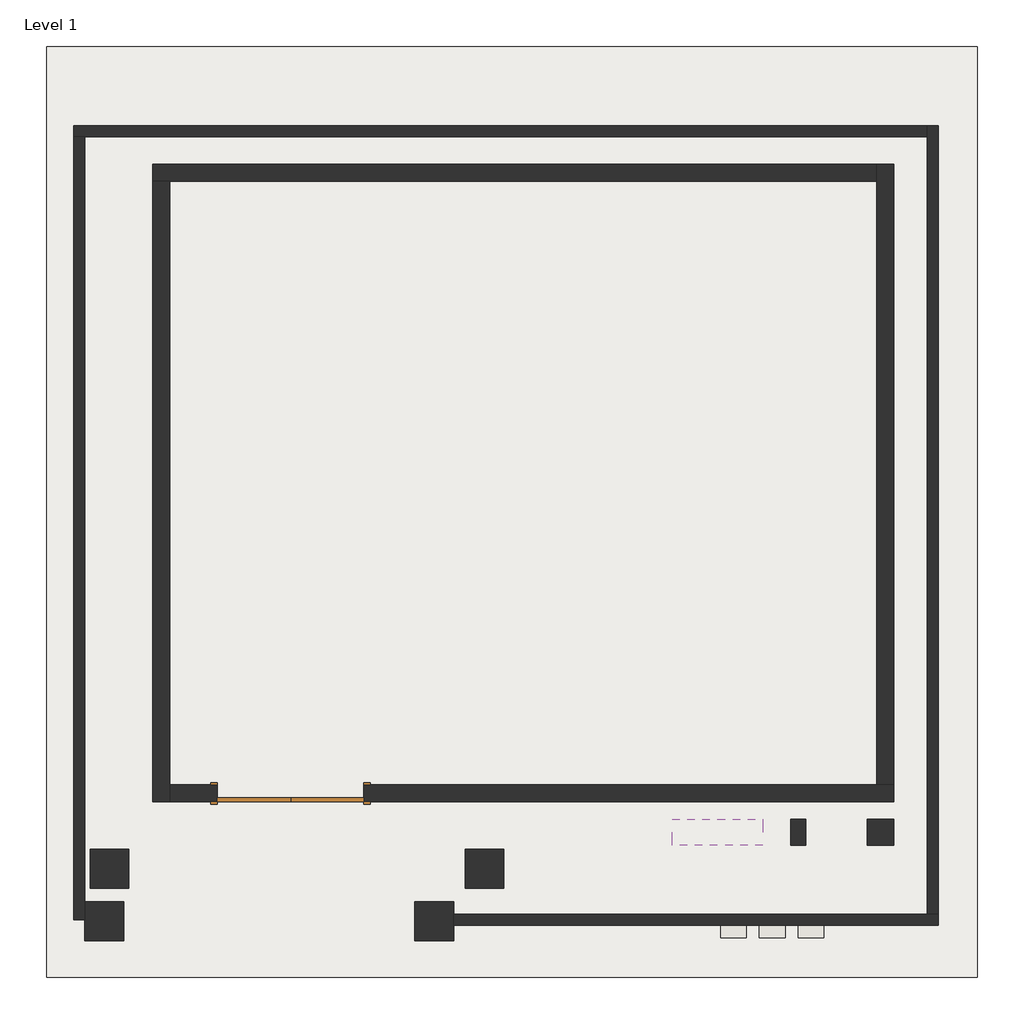
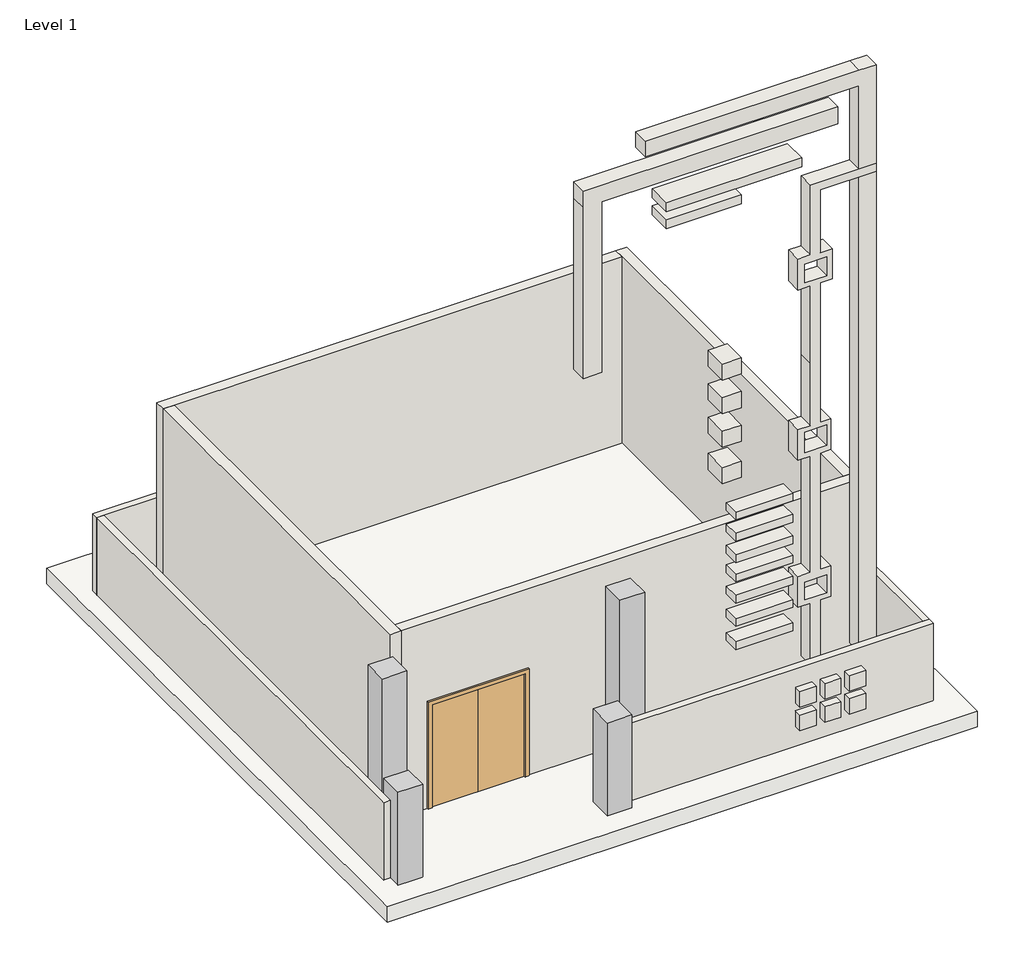
# One storey: 12 walls, 4 columns, 1 door, 1 slab.
"""IFC4 building model written with IfcOpenShell, lengths in millimetres."""

from ifc_helpers import new_model, si_unit, frame, origin, origin_with_axes, place, context, project, spatial, polyline, outline, extrude, faceted_brep, transform, mapped, element, save
from components import column_ce396696, door_aae36eb6, walls_1_walls_1_5a20c518, walls_5_walls_5_fc3546cb, walls_6_walls_6_ffd2a55d, walls_7_walls_7_e8c1ea63

model = new_model("IFC4")

# Units and contexts
model_context = context("Model", 3, world=origin())
ifc_project = project(units=[si_unit("LENGTHUNIT", "METRE", prefix="MILLI")], contexts=[model_context])

# Site, building, storey
site = spatial("IfcSite", under=ifc_project)
building = spatial("IfcBuilding", under=site)
storey = spatial("IfcBuildingStorey", under=building, Name="Level 1", Elevation=0.0)

# Columns
placement = place(None, origin())
element("IfcColumn", 1, ObjectType="Rectangular Column : 18\" x 18\"", at=placement, inside=storey, context=model_context, shape_type="SweptSolid", body=[
    extrude(outline(polyline([(-5771.1093643, 1455.1827135), (-5771.1093643, 997.9827135), (-6228.3093643, 997.9827135), (-6228.3093643, 1455.1827135), (-5771.1093643, 1455.1827135)])), origin_with_axes(), (0.0, 0.0, 1.0), 3657.6),
])
element("IfcColumn", 2, ObjectType="Rectangular Column : 18\" x 18\"", at=placement, inside=storey, context=model_context, shape_type="Brep", body=[
    faceted_brep([(-10255.0909085, 837.6674273, 1828.8), (-10712.2909085, 837.6674273, 1828.8), (-10712.2909085, 380.4674273, 1828.8), (-10255.0909085, 380.4674273, 1828.8), (-10255.0909085, 837.6674273, 0.0), (-10255.0909085, 380.4674273, 0.0), (-10712.2909085, 380.4674273, 0.0), (-10712.2909085, 624.7297756, 0.0), (-10712.2909085, 837.6674273, 0.0)], [[[0, 1, 2, 3]], [[4, 5, 6, 7, 8]], [[1, 0, 4, 8]], [[2, 1, 8, 7, 6]], [[3, 2, 6, 5]], [[0, 3, 5, 4]]]),
])
element("IfcColumn", 3, ObjectType="Rectangular Column : 18\" x 18\"", at=placement, inside=storey, context=model_context, shape_type="Brep", body=[
    faceted_brep([(-6365.0284004, 837.6674273, 1828.8), (-6822.2284004, 837.6674273, 1828.8), (-6822.2284004, 380.4674273, 1828.8), (-6365.0284004, 380.4674273, 1828.8), (-6365.0284004, 837.6674273, 0.0), (-6365.0284004, 689.4718041, 0.0), (-6365.0284004, 562.4718041, 0.0), (-6365.0284004, 380.4674273, 0.0), (-6822.2284004, 380.4674273, 0.0), (-6822.2284004, 837.6674273, 0.0)], [[[0, 1, 2, 3]], [[4, 5, 6, 7, 8, 9]], [[1, 0, 4, 9]], [[2, 1, 9, 8]], [[3, 2, 8, 7]], [[0, 3, 7, 6, 5, 4]]]),
])
column_shape = column_ce396696(model_context)
element("IfcColumn", 4, ObjectType="Rectangular Column : 18\" x 18\"", at=placement, inside=storey, context=model_context, shape_type="MappedRepresentation", body=[
    mapped(column_shape, transform((-10419.3093643, 1226.5827135, 0.0), x_axis=(1.0, 0.0, 0.0), y_axis=(0.0, 1.0, 0.0), z_axis=(0.0, 0.0, 1.0))),
])

# Door
door_shape = door_aae36eb6(model_context)
element("IfcDoor", 5, ObjectType="Door-Double-Flush_Panel : 68\" x 80\"", at=placement, inside=storey, context=model_context, shape_type="MappedRepresentation", body=[
    mapped(door_shape, transform((-8285.7093643, 2115.5827135, 0.0), x_axis=(-1.0, 0.0, 0.0), y_axis=(0.0, -1.0, 0.0), z_axis=(0.0, 0.0, 1.0))),
])

# Slab
element("IfcSlab", 6, ObjectType="Generic - 12\"", at=placement, inside=storey, context=model_context, shape_type="SweptSolid", body=[
    extrude(outline(polyline([(-189.3944008, 10918.5162537), (-189.3944008, -54.2837463), (-11162.1944008, -54.2837463), (-11162.1944008, 10918.5162537), (-189.3944008, 10918.5162537)])), frame((0.0, 0.0, -304.8), z_axis=(0.0, 0.0, 1.0), x_axis=(1.0, 0.0, 0.0)), (0.0, 0.0, 1.0), 304.8),
])

# Walls
element("IfcWall", 7, ObjectType="Generic - 5\"", at=placement, inside=storey, context=model_context, shape_type="Brep", body=[
    faceted_brep([(-10839.2909085, 9857.6297756, 0.0), (-10712.2909085, 9857.6297756, 0.0), (-780.8909085, 9857.6297756, 0.0), (-780.8909085, 9857.6297756, 1524.0), (-10712.2909085, 9857.6297756, 1524.0), (-10839.2909085, 9857.6297756, 1524.0), (-10839.2909085, 9984.6297756, 0.0), (-10839.2909085, 9984.6297756, 1524.0), (-780.8909085, 9984.6297756, 1524.0), (-780.8909085, 9984.6297756, 0.0)], [[[0, 1, 2, 3, 4, 5]], [[6, 7, 8, 9]], [[2, 1, 0, 6, 9]], [[5, 4, 3, 8, 7]], [[0, 5, 7, 6]], [[3, 2, 9, 8]]]),
])
element("IfcWall", 8, ObjectType="Generic - 5\"", at=placement, inside=storey, context=model_context, shape_type="Brep", body=[
    faceted_brep([(-10712.2909085, 624.7297756, 0.0), (-10712.2909085, 837.6674273, 0.0), (-10712.2909085, 9857.6297756, 0.0), (-10712.2909085, 9857.6297756, 1524.0), (-10712.2909085, 624.7297756, 1524.0), (-10839.2909085, 624.7297756, 0.0), (-10839.2909085, 624.7297756, 1524.0), (-10839.2909085, 9857.6297756, 1524.0), (-10839.2909085, 9857.6297756, 0.0)], [[[0, 1, 2, 3, 4]], [[5, 6, 7, 8]], [[2, 1, 0, 5, 8]], [[4, 3, 7, 6]], [[0, 4, 6, 5]], [[3, 2, 8, 7]]]),
])
element("IfcWall", 9, ObjectType="Generic - 5\"", at=placement, inside=storey, context=model_context, shape_type="Brep", body=[
    faceted_brep([(-653.8909085, 689.4718041, 0.0), (-780.8909085, 689.4718041, 0.0), (-6365.0284004, 689.4718041, 0.0), (-6365.0284004, 689.4718041, 1524.0), (-780.8909085, 689.4718041, 1524.0), (-653.8909085, 689.4718041, 1524.0), (-653.8909085, 562.4718041, 0.0), (-653.8909085, 562.4718041, 1524.0), (-6365.0284004, 562.4718041, 1524.0), (-6365.0284004, 562.4718041, 0.0)], [[[0, 1, 2, 3, 4, 5]], [[6, 7, 8, 9]], [[2, 1, 0, 6, 9]], [[3, 2, 9, 8]], [[5, 4, 3, 8, 7]], [[0, 5, 7, 6]]]),
])
element("IfcWall", 10, ObjectType="Generic - 5\"", at=placement, inside=storey, context=model_context, shape_type="Brep", body=[
    faceted_brep([(-780.8909085, 9984.6297756, 0.0), (-780.8909085, 9857.6297756, 0.0), (-780.8909085, 689.4718041, 0.0), (-780.8909085, 689.4718041, 1524.0), (-780.8909085, 9857.6297756, 1524.0), (-780.8909085, 9984.6297756, 1524.0), (-653.8909085, 9984.6297756, 0.0), (-653.8909085, 9984.6297756, 1524.0), (-653.8909085, 689.4718041, 1524.0), (-653.8909085, 689.4718041, 0.0)], [[[0, 1, 2, 3, 4, 5]], [[6, 7, 8, 9]], [[2, 1, 0, 6, 9]], [[5, 4, 3, 8, 7]], [[0, 5, 7, 6]], [[3, 2, 9, 8]]]),
])
element("IfcWall", 11, ObjectType="Generic - 8\"", at=placement, inside=storey, context=model_context, shape_type="Brep", body=[
    faceted_brep([(-9911.3093643, 9329.1827135, 0.0), (-9708.1093643, 9329.1827135, 0.0), (-1376.9093643, 9329.1827135, 0.0), (-1376.9093643, 9329.1827135, 3657.6), (-9708.1093643, 9329.1827135, 3657.6), (-9911.3093643, 9329.1827135, 3657.6), (-9911.3093643, 9532.3827135, 0.0), (-9911.3093643, 9532.3827135, 3657.6), (-1376.9093643, 9532.3827135, 3657.6), (-1376.9093643, 9532.3827135, 0.0)], [[[0, 1, 2, 3, 4, 5]], [[6, 7, 8, 9]], [[2, 1, 0, 6, 9]], [[0, 5, 7, 6]], [[3, 2, 9, 8]], [[5, 4, 3, 8, 7]]]),
])
element("IfcWall", 12, ObjectType="Generic - 8\"", at=placement, inside=storey, context=model_context, shape_type="Brep", body=[
    faceted_brep([(-9708.1093643, 2013.9827135, 0.0), (-9708.1093643, 2217.1827135, 0.0), (-9708.1093643, 9329.1827135, 0.0), (-9708.1093643, 9329.1827135, 3657.6), (-9708.1093643, 2217.1827135, 3657.6), (-9708.1093643, 2013.9827135, 3657.6), (-9911.3093643, 2013.9827135, 0.0), (-9911.3093643, 2013.9827135, 3657.6), (-9911.3093643, 9329.1827135, 3657.6), (-9911.3093643, 9329.1827135, 0.0)], [[[0, 1, 2, 3, 4, 5]], [[6, 7, 8, 9]], [[2, 1, 0, 6, 9]], [[0, 5, 7, 6]], [[3, 2, 9, 8]], [[5, 4, 3, 8, 7]]]),
])
element("IfcWall", 13, ObjectType="Generic - 8\"", at=placement, inside=storey, context=model_context, shape_type="Brep", body=[
    faceted_brep([(-1173.7093643, 2217.1827135, 3657.6), (-1173.7093643, 2217.1827135, 0.0), (-1376.9093643, 2217.1827135, 0.0), (-7422.1093643, 2217.1827135, 0.0), (-7422.1093643, 2217.1827135, 2032.0), (-9149.3093643, 2217.1827135, 2032.0), (-9149.3093643, 2217.1827135, 0.0), (-9708.1093643, 2217.1827135, 0.0), (-9708.1093643, 2217.1827135, 3657.6), (-1376.9093643, 2217.1827135, 3657.6), (-1173.7093643, 2013.9827135, 0.0), (-1173.7093643, 2013.9827135, 3657.6), (-5542.5093643, 2013.9827135, 3657.6), (-9708.1093643, 2013.9827135, 3657.6), (-9708.1093643, 2013.9827135, 0.0), (-9149.3093643, 2013.9827135, 0.0), (-9149.3093643, 2013.9827135, 2032.0), (-7422.1093643, 2013.9827135, 2032.0), (-7422.1093643, 2013.9827135, 0.0)], [[[0, 1, 2, 3, 4, 5, 6, 7, 8, 9]], [[10, 11, 12, 13, 14, 15, 16, 17, 18]], [[1, 10, 18, 3, 2]], [[14, 7, 6, 15]], [[1, 0, 11, 10]], [[8, 7, 14, 13]], [[11, 0, 9, 8, 13, 12]], [[5, 16, 15, 6]], [[16, 5, 4, 17]], [[17, 4, 3, 18]]]),
])
element("IfcWall", 14, ObjectType="Generic - 8\"", at=placement, inside=storey, context=model_context, shape_type="Brep", body=[
    faceted_brep([(-1376.9093643, 9532.3827135, 0.0), (-1376.9093643, 9329.1827135, 0.0), (-1376.9093643, 2217.1827135, 0.0), (-1376.9093643, 2217.1827135, 3657.6), (-1376.9093643, 9329.1827135, 3657.6), (-1376.9093643, 9532.3827135, 3657.6), (-1173.7093643, 9532.3827135, 0.0), (-1173.7093643, 9532.3827135, 3657.6), (-1173.7093643, 2217.1827135, 3657.6), (-1173.7093643, 2217.1827135, 0.0)], [[[0, 1, 2, 3, 4, 5]], [[6, 7, 8, 9]], [[2, 1, 0, 6, 9]], [[0, 5, 7, 6]], [[3, 2, 9, 8]], [[5, 4, 3, 8, 7]]]),
])
walls_1_walls_1_shape = walls_1_walls_1_5a20c518(model_context)
element("IfcWall", 15, ObjectType="Walls 1 : Walls 1", at=placement, inside=storey, context=model_context, shape_type="MappedRepresentation", body=[
    mapped(walls_1_walls_1_shape, transform((0.0, 0.0, 0.0), x_axis=(1.0, 0.0, 0.0), y_axis=(0.0, 1.0, 0.0), z_axis=(0.0, 0.0, 1.0))),
])
walls_5_walls_5_shape = walls_5_walls_5_fc3546cb(model_context)
element("IfcWall", 16, ObjectType="Walls 5 : Walls 5", at=placement, inside=storey, context=model_context, shape_type="MappedRepresentation", body=[
    mapped(walls_5_walls_5_shape, transform((0.0, 0.0, 0.0), x_axis=(1.0, 0.0, 0.0), y_axis=(0.0, 1.0, 0.0), z_axis=(0.0, 0.0, 1.0))),
])
walls_6_walls_6_shape = walls_6_walls_6_ffd2a55d(model_context)
element("IfcWall", 17, ObjectType="Walls 6 : Walls 6", at=placement, inside=storey, context=model_context, shape_type="MappedRepresentation", body=[
    mapped(walls_6_walls_6_shape, transform((0.0, 0.0, 0.0), x_axis=(1.0, 0.0, 0.0), y_axis=(0.0, 1.0, 0.0), z_axis=(0.0, 0.0, 1.0))),
])
walls_7_walls_7_shape = walls_7_walls_7_e8c1ea63(model_context)
element("IfcWall", 18, ObjectType="Walls 7 : Walls 7", at=placement, inside=storey, context=model_context, shape_type="MappedRepresentation", body=[
    mapped(walls_7_walls_7_shape, transform((0.0, 0.0, 0.0), x_axis=(1.0, 0.0, 0.0), y_axis=(0.0, 1.0, 0.0), z_axis=(0.0, 0.0, 1.0))),
])

save(model, "model.ifc")

# Revit data of these elements
# Type "Rectangular Column : 18\" x 18\""
#   Assembly Code = "B1010200"
#   Depth = 1' - 6"
#   Offset Base = 0' - 0"
#   Offset Top = 0' - 0"
#   Width = 1' - 6"
#   Material = none
# Type "Door-Double-Flush_Panel : 68\" x 80\""
#   Type Mark = "8"
#   Construction Type Id = "DOOR"
#   Assembly Code = "C1020"
#   Analytic Construction = "Wooden"
#   Thickness = 0' - 2"
#   Thermal Resistance (R) = 2.5876 (h·ft²·°F)/BTU
#   Swing Angle [instance default] = 90.00°
#   Panel Width = 2' - 10"
#   Heat Transfer Coefficient (U) = 0.3865 BTU/(h·ft²·°F)
#   Height = 6' - 8"
#   Trim Projection Ext = 0' - 1"
#   Trim Projection Int = 0' - 1"
#   Trim Width = 0' - 3"
#   Width = 5' - 8"
#   Define Thermal Properties by = 1
#   Panel Material = Wood - Birch - Solid Stained Light Low Gloss
#   Trim Material = Paint - Sienna
#   Visual Light Transmittance = 0
#   Solar Heat Gain Coefficient = 0
#   Function = (empty or 0)
#   Wall Closure = (empty or 0)
# Type "Generic - 12\""
#   Assembly Code = "B1010"
#   Function = 0
#   Layers, outside or top first: 1' - 0" no material (function 1)
# Type "Generic - 5\""
#   Assembly Code = "B2010"
#   Layers, outside or top first: 0' - 5" no material (function 1)
# Type "Generic - 8\""
#   Assembly Code = "B2010"
#   Layers, outside or top first: 0' - 8" no material (function 1)
# Elements 1, 4 (IfcColumn, "Rectangular Column : 18\" x 18\"")
#   Phase Created = New Construction
# Elements 2, 3 (IfcColumn, "Rectangular Column : 18\" x 18\"")
#   Phase Created = New Construction
#   Materials on its faces: "Default Wall"
# Element 5 (IfcDoor, "Door-Double-Flush_Panel : 68\" x 80\"")
#   Swing Angle = 90.00°
#   Phase Created = New Construction
#   Materials on its faces: "Paint - Sienna", "Wood - Birch - Solid Stained Light Low Gloss"
# Element 6 (IfcSlab, "Generic - 12\"")
#   Height Offset From Level = 0' - 0"
#   Phase Created = New Construction
#   Materials on its faces: "Default Floor"
# Elements 7, 8, 9, 10 (IfcWall, "Generic - 5\"")
#   Top Offset = -7' - 0"
#   Base Offset = 0' - 0"
#   wall height = 5' - 0"
#   Phase Created = New Construction
#   Base Constraint = Level 1
#   Top Constraint = Level 2
#   Materials on its faces: "Default Wall"
# Elements 11, 12, 13, 14 (IfcWall, "Generic - 8\"")
#   Top Offset = 0' - 0"
#   Base Offset = 0' - 0"
#   Unconnected Height = 12' - 0"
#   wall height = 12' - 0"
#   Phase Created = New Construction
#   Base Constraint = Level 1
#   Materials on its faces: "Default Wall"
# Element 15 (IfcWall, "Walls 1 : Walls 1")
#   Phase Created = New Construction
#   Materials on its faces: "Default Wall"
# Element 16 (IfcWall, "Walls 5 : Walls 5")
#   Phase Created = New Construction
#   Materials on its faces: "Default Wall"
# Element 17 (IfcWall, "Walls 6 : Walls 6")
#   Phase Created = New Construction
#   Materials on its faces: "Default Wall"
# Element 18 (IfcWall, "Walls 7 : Walls 7")
#   Phase Created = New Construction
#   Materials on its faces: "Default Wall"
# Materials
#   "Wood - Birch - Solid Stained Light Low Gloss": class "Wood", colour RGB 210 159 95, transparency 0, Cost = 0
#   "Paint - Sienna": colour RGB 118 70 51, transparency 0, Cost = 0
#   "Default Wall": colour RGB 128 128 128, transparency 0
#   "Default Floor": colour RGB 128 128 128, transparency 0
